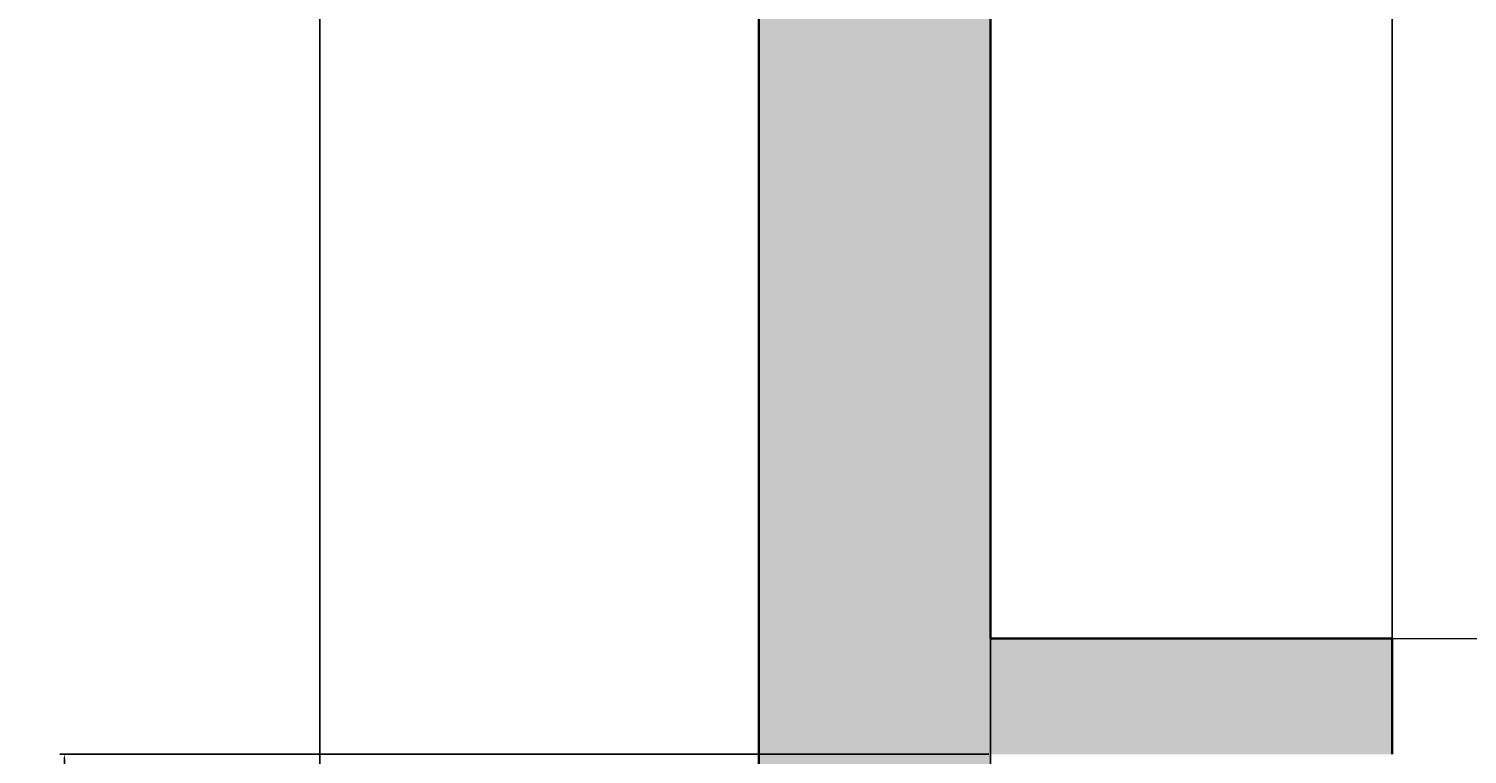
# Model space of a CAD drawing. Units: inches. Extents: x -5 to 330, y -522 to 40.
# Tile 11 of 23: x -5 to 51, y -297 to -269. Entities that reach past the tile are written whole.
import ezdxf

# ---------------------------------------------------------------- set-up
doc = ezdxf.new("R2010")
doc.units = ezdxf.units.IN
doc.header["$MEASUREMENT"] = 0
doc.linetypes.add('ACAD_ISO02W100', pattern=[15, 12, -3])
for name, color, linetype, lineweight in [('A-ANNO-DIMS', 2, 'Continuous', 18), ('A-WALL', 7, 'Continuous', 35), ('A-WALL-OVHD', 8, 'ACAD_ISO02W100', 18)]:
    doc.layers.add(name, color=color, linetype=linetype, lineweight=lineweight)
doc.layers.add('A-WALL-PATT', color=18, linetype='Continuous', lineweight=13, true_color=0x000000)
doc.styles.get("Standard").update_dxf_attribs({"font": 'arial.ttf'})
doc.dimstyles.get("Standard").update_dxf_attribs({"dimtxt": 0.18, "dimasz": 0.18, "dimexe": 0.18, "dimexo": 0.0625, "dimgap": 0.09, "dimtad": 0, "dimtih": 1, "dimtoh": 1, "dimdec": 0, "dimzin": 0, "dimdsep": 46, "dimlunit": 3, "dimtxsty": 'Standard', "dimcen": 0.09, "dimadec": 0, "dimazin": 0, "dimtfac": 1, "dimtdec": 0, "dimtofl": 0, "dimtmove": 0, "dimatfit": 3, "dimfxl": 1, "dimtolj": 1, "dimtzin": 0, "dimarcsym": 0})

# ---------------------------------------------------------------- blocks, each defined once
blk = doc.blocks.new('*D2')
at = {"layer": 'A-ANNO-DIMS', "color": 0, "lineweight": -2, "transparency": 16777216}
for p, q in [((23.447, 12.356), (6.274, 12.356)), ((6.454, 12.176), (6.454, -203.738)), ((6.454, -425.964), (6.454, -210.049)), ((23.447, -426.144), (6.274, -426.144))]:
    blk.add_line(p, q, dxfattribs=at)
at = {"layer": 'A-ANNO-DIMS', "color": 0, "transparency": 16777216}
for points in [[(6.424, 12.176), (6.484, 12.176), (6.454, 12.356)], [(6.424, -425.964), (6.484, -425.964), (6.454, -426.144)]]:
    blk.add_solid(points, dxfattribs=at)
at = {"layer": 'Defpoints', "color": 0, "transparency": 16777216}
for p in [(23.51, 12.356), (6.454, -426.144), (23.51, -426.144)]:
    blk.add_point(p, dxfattribs=at)
at = {"layer": 'A-ANNO-DIMS', "color": 0, "transparency": 16777216, "insert": (6.454, -206.894), "char_height": 6, "attachment_point": 5}
blk.add_mtext('\\A1;36\'-7"', dxfattribs=at)
blk = doc.blocks.new('*D40')
at = {"layer": 'A-ANNO-DIMS', "color": 0, "lineweight": -2, "transparency": 16777216}
for p, q in [((32.51, -246.706), (32.51, -522.309)), ((79.01, -246.706), (79.01, -522.309)), ((32.69, -522.129), (55.151, -522.129)), ((78.83, -522.129), (56.369, -522.129))]:
    blk.add_line(p, q, dxfattribs=at)
at = {"layer": 'A-ANNO-DIMS', "color": 0, "transparency": 16777216}
for points in [[(32.69, -522.099), (32.69, -522.159), (32.51, -522.129)], [(78.83, -522.099), (78.83, -522.159), (79.01, -522.129)]]:
    blk.add_solid(points, dxfattribs=at)
at = {"layer": 'Defpoints', "color": 0, "transparency": 16777216}
for p in [(32.51, -246.644), (79.01, -246.644), (79.01, -522.129)]:
    blk.add_point(p, dxfattribs=at)
at = {"layer": 'A-ANNO-DIMS', "color": 0, "transparency": 16777216, "insert": (55.76, -522.129), "char_height": 0.18, "attachment_point": 5}
blk.add_mtext('\\A1;3\'-10 1/2"', dxfattribs=at)
blk = doc.blocks.new('*D43')
at = {"layer": 'A-ANNO-DIMS', "color": 0, "lineweight": -2, "transparency": 16777216}
for p, q in [((32.51, -297.081), (32.51, 39.521)), ((32.69, 39.341), (39.789, 39.341)), ((47.949, 39.341), (40.85, 39.341)), ((48.129, -297.081), (48.129, 39.521))]:
    blk.add_line(p, q, dxfattribs=at)
at = {"layer": 'A-ANNO-DIMS', "color": 0, "transparency": 16777216}
for points in [[(32.69, 39.371), (32.69, 39.311), (32.51, 39.341)], [(47.949, 39.371), (47.949, 39.311), (48.129, 39.341)]]:
    blk.add_solid(points, dxfattribs=at)
at = {"layer": 'Defpoints', "color": 0, "transparency": 16777216}
for p in [(48.129, 39.341), (32.51, -297.144), (48.129, -297.144)]:
    blk.add_point(p, dxfattribs=at)
at = {"layer": 'A-ANNO-DIMS', "color": 0, "transparency": 16777216, "insert": (40.319, 39.341), "char_height": 0.18, "attachment_point": 5}
blk.add_mtext('\\A1;1\'-3 1/2"', dxfattribs=at)
blk = doc.blocks.new('*D47')
at = {"layer": 'A-ANNO-DIMS', "color": 0, "lineweight": -2, "transparency": 16777216}
for p, q in [((32.447, -297.144), (-3.655, -297.144)), ((-3.475, -297.324), (-3.475, -300.609)), ((-3.475, -304.261), (-3.475, -300.975)), ((33.036, -304.441), (-3.655, -304.441))]:
    blk.add_line(p, q, dxfattribs=at)
at = {"layer": 'A-ANNO-DIMS', "color": 0, "transparency": 16777216}
for points in [[(-3.505, -297.324), (-3.445, -297.324), (-3.475, -297.144)], [(-3.505, -304.261), (-3.445, -304.261), (-3.475, -304.441)]]:
    blk.add_solid(points, dxfattribs=at)
at = {"layer": 'Defpoints', "color": 0, "transparency": 16777216}
for p in [(32.51, -297.144), (-3.475, -304.441), (33.099, -304.441)]:
    blk.add_point(p, dxfattribs=at)
at = {"layer": 'A-ANNO-DIMS', "color": 0, "transparency": 16777216, "insert": (-3.475, -300.792), "char_height": 0.18, "attachment_point": 5}
blk.add_mtext('\\A1;0\'-7 1/2"', dxfattribs=at)

msp = doc.modelspace()

# ---------------------------------------------------------------- hatches: boundary and pattern name
at = {"layer": 'A-WALL-PATT'}
h = msp.add_hatch(color=256, dxfattribs=at)
h.dxf.hatch_style = 1
h.paths.add_polyline_path([(164.01, -44.152), (159.51, -44.152), (159.51, -153.144), (164.01, -153.144)], flags=17)
h.paths.add_polyline_path([(224.01, -188.144), (272.01, -188.144), (272.01, -218.144), (260.01, -218.144), (260.01, -222.644), (272.01, -222.644), (272.01, -292.644), (159.01, -292.644), (159.01, -297.144), (272.01, -297.144), (272.01, -417.144), (245.51, -417.144), (245.51, -426.144), (272.01, -426.144), (272.01, -495.144), (281.01, -495.144), (281.01, 12.356), (23.51, 12.356), (23.51, -426.144), (62.918, -426.144), (62.918, -417.144), (32.51, -417.144), (32.51, -297.144), (48.129, -297.144), (48.129, -292.644), (32.51, -292.644), (32.51, -140.644), (133.51, -140.644), (133.51, -131.644), (32.51, -131.644), (32.51, 3.356), (159.51, 3.356), (164.01, 3.356), (220.01, 3.356), (224.51, 3.356), (272.01, 3.356), (272.01, -179.144), (159.51, -179.144), (159.51, -188.144), (219.51, -188.144), (219.51, -266.644), (224.01, -266.644), (224.01, -222.644), (236.01, -222.644), (236.01, -218.144), (224.01, -218.144)])
h.paths.add_polyline_path([(133.01, -292.644), (128.51, -292.644), (128.51, -297.144), (128.51, -417.144), (122.918, -417.144), (122.918, -426.144), (133.01, -426.144)], flags=17)
h.paths.add_polyline_path([(185.51, -417.144), (159.01, -417.144), (159.01, -426.144), (185.51, -426.144)], flags=17)
h.paths.add_polyline_path([(133.51, -140.644), (129.01, -140.644), (129.01, -246.644), (133.51, -246.644)], flags=17)
h.paths.add_polyline_path([(246.01, -48.644), (224.51, -48.644), (224.51, -27.627), (220.01, -27.627), (220.01, -48.644), (198.604, -48.644), (198.604, -53.144), (246.01, -53.144)], flags=17)

# ---------------------------------------------------------------- linework, layer by layer
at = {"layer": 'A-WALL'}
for p, q in [((23.51, 12.356), (23.51, -495.144)), ((32.51, -140.644), (32.51, -292.644)), ((32.51, -292.644), (48.129, -292.644)), ((48.129, -292.644), (48.129, -297.144))]:
    msp.add_line(p, q, dxfattribs=at)
at = {"layer": 'A-WALL-OVHD'}
msp.add_line((48.129, -292.644), (128.51, -292.644), dxfattribs=at)

# ---------------------------------------------------------------- dimensions: what is measured, and where the dimension line sits
at = {"layer": 'A-ANNO-DIMS'}
for base, p1, p2, picture, middle in [((48.129, 39.341), (32.51, -297.144), (48.129, -297.144), '*D43', (40.319, 39.341)), ((79.01, -522.129), (32.51, -246.644), (79.01, -246.644), '*D40', (55.76, -522.129))]:
    dim = msp.add_linear_dim(base=base, p1=p1, p2=p2, dimstyle='Standard', override={"dimdec": 1, "dimlfac": 1, "dimrnd": 0, "dimzin": 1, "dimdsep": 46, "dimlunit": 4, "dimfrac": 2}, dxfattribs=at)
    dim.commit()
    dim.dimension.update_dxf_attribs({"geometry": picture, "text_midpoint": middle})
for base, p1, p2, override, picture, middle in [((6.454321893, -426.143582029), (23.509888577, 12.356417971), (23.509888577, -426.143582029), {"dimtxt": 6, "dimclrd": 0, "dimclre": 0, "dimclrt": 0}, '*D2', (6.454321893, -206.893582029)), ((-3.475, -304.441), (32.51, -297.144), (33.099, -304.441), {"dimdec": 1, "dimlfac": 1, "dimrnd": 0, "dimzin": 1, "dimdsep": 46, "dimlunit": 4, "dimfrac": 2}, '*D47', (-3.475, -300.792))]:
    dim = msp.add_linear_dim(base=base, p1=p1, p2=p2, angle=90, dimstyle='Standard', override=override, dxfattribs=at)
    dim.commit()
    dim.dimension.update_dxf_attribs({"geometry": picture, "text_midpoint": middle})

doc.saveas('drawing.dxf')
